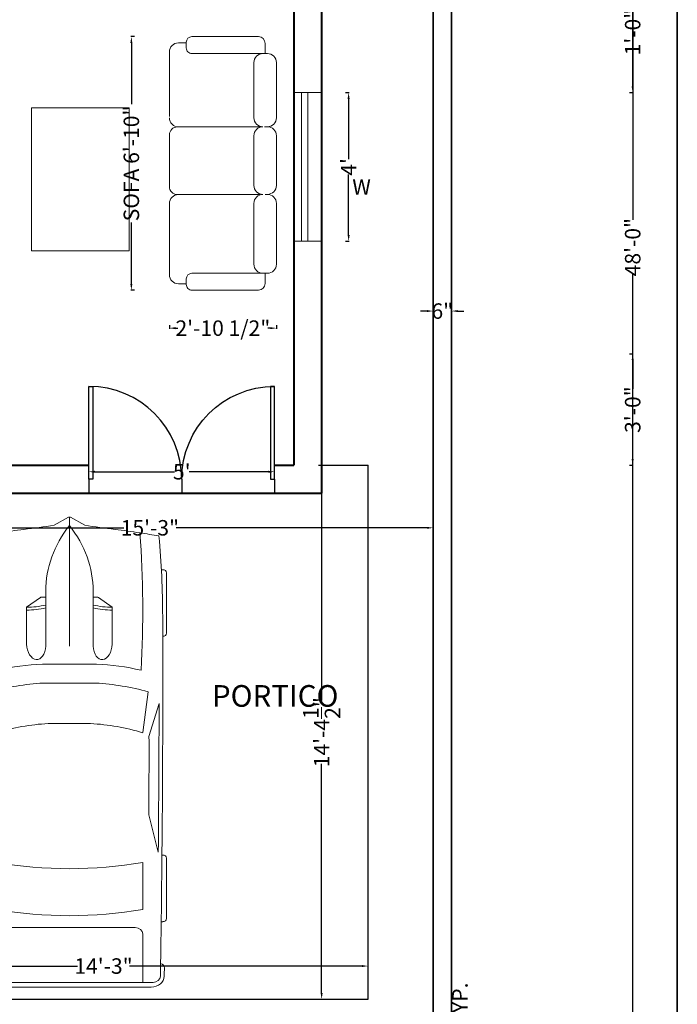
# Model space of a CAD drawing. Units: inches. Extents: x -231 to 349, y -511 to 252.
# Tile 4 of 6: x 136 to 349, y -351 to -33. Entities that reach past the tile are written whole.
import ezdxf

# ---------------------------------------------------------------- set-up
doc = ezdxf.new("R2010")
doc.units = ezdxf.units.IN
doc.header["$MEASUREMENT"] = 0
for name, color, linetype, lineweight in [('A-ANNO-DIMS', 7, 'Continuous', 18), ('A-ANNO-TEXT', 7, 'Continuous', 18), ('A-ANNO-TTLB', 7, 'Continuous', 35), ('A-AREA-IDEN', 7, 'Continuous', 25), ('A-FLOR', 7, 'Continuous', 25), ('A-FURN', 8, 'Continuous', 18), ('A-GLAZ', 177, 'Continuous', 20), ('A-WALL', 7, 'Continuous', 40), ('C-PARK-VEHI', 8, 'Continuous', 13), ('C-PROP', 7, 'Continuous', 35), ('DOOR', 42, 'Continuous', 25)]:
    doc.layers.add(name, color=color, linetype=linetype, lineweight=lineweight)
doc.styles.get("Standard").update_dxf_attribs({"font": 'arial.ttf'})
doc.dimstyles.get("Standard").update_dxf_attribs({"dimtxt": 5, "dimasz": 2, "dimexe": 0.18, "dimexo": 0.0625, "dimgap": 0.09, "dimtad": 0, "dimzin": 0, "dimdsep": 46, "dimlunit": 4, "dimtxsty": 'Standard', "dimcen": 0.09, "dimadec": 0, "dimazin": 0, "dimtfac": 1, "dimtofl": 0, "dimtmove": 0, "dimatfit": 3, "dimfxl": 1, "dimfxlon": 1, "dimtolj": 1, "dimtzin": 0, "dimarcsym": 0})

# ---------------------------------------------------------------- blocks, each defined once
blk = doc.blocks.new('*U2')
for p, q in [((0, 0), (0, -6)), ((40, 0), (40, -6))]:
    blk.add_line(p, q)
blk.add_lwpolyline([(0, 0), (0, 40), (1.75, 40), (1.75, 0)], close=True)
blk.add_arc((0, 0), 40, 0, 90)
blk = doc.blocks.new('*U7')
for p, q in [((21.1, 37.41), (21.1, 36.83)), ((46.55, 38.89), (22.35, 38.89)), ((47.8, 37.39), (47.8, 37.41)), ((87.99, 31.87), (74.76, 35.92)), ((134.31, 35.6), (119.29, 31.78)), ((135.45, 37.07), (135.45, 37.41)), ((136.7, 38.89), (160.9, 38.89)), ((162.15, 37.41), (162.15, 36.77)), ((186.47, -33.5), (186.47, 33.5)), ((188.4, -32.76), (188.4, 32.76)), ((70.03, 31.54), (86.41, 29.35)), ((138.42, 29.35), (157.25, 29.35)), ((186.47, 29.35), (167.01, 29.35)), ((164.52, 26.39), (164.52, -26.39)), ((32.27, 11.63), (36.13, 17.17)), ((36.13, 17.17), (50.94, 17.17)), ((29.77, 9.51), (51.68, 9.51)), ((32.12, 9.51), (32.12, 11.15)), ((58.92, -10.77), (58.92, 10.77)), ((66.55, -10.53), (66.55, 10.53)), ((82.74, 8.5), (82.74, -8.5)), ((186.47, -10.53), (186.47, 10.53)), ((3.27, 6.13), (0.1, 0.41)), ((0, 0), (51.68, 0)), ((0.1, -0.41), (3.27, -6.13)), ((29.77, -9.51), (51.68, -9.51)), ((32.12, -9.51), (32.12, -11.15)), ((32.27, -11.63), (36.13, -17.17)), ((36.13, -17.17), (50.94, -17.17)), ((86.41, -29.35), (70.03, -31.54)), ((157.25, -29.35), (138.42, -29.35)), ((167.01, -29.35), (186.47, -29.35)), ((87.99, -31.87), (74.76, -35.92)), ((134.31, -35.6), (119.29, -31.78)), ((21.1, -37.41), (21.1, -36.83)), ((46.55, -38.89), (22.35, -38.89)), ((47.8, -37.39), (47.8, -37.41)), ((135.45, -37.07), (135.45, -37.41)), ((136.7, -38.89), (160.9, -38.89)), ((162.15, -37.41), (162.15, -36.77))]:
    blk.add_line(p, q)
for centre, major_axis, ratio, start_param, end_param in [((266.03, -27.52), (0, 313.31), 0.842304, 1.367076, 1.39176), ((41.19, -490.86), (0, 528.23), 0.842304, 0.00281, 0.075598), ((22.35, 37.41), (0, -1.48), 0.842304, 3.141593, 4.712389), ((64.48, -10555.62), (0, 10593.03), 0.842304, -0.013397, 0.002797), ((46.55, 37.41), (0, 1.48), 0.842304, -1.570796, 0), ((64.48, -10555.62), (0, -10591.55), 0.842304, 3.133765, 3.140441), ((136.7, 37.41), (0, -1.48), 0.842304, 3.141593, 4.712389), ((160.9, 37.41), (0, 1.48), 0.842304, -1.570796, 0), ((180.63, 35.84), (0, 2.22), 0.842304, -0.013017, 1.249894), ((64.48, -10556.36), (0, 10595.31), 0.842304, -0.013397, -0.013017), ((183.98, 33.5), (0, -2.96), 0.842304, 1.570796, 3.128196), ((183.98, 32.76), (0, -5.25), 0.842304, 1.570796, 3.128196), ((95.79, -3666.35), (0, -3698.24), 0.842304, 3.134049, 3.144098), ((259.18, -27.52), (0, -305.3), 0.842304, 4.528606, 4.561838), ((37.47, -593.96), (0, -623.33), 0.842304, 3.096046, 3.200911), ((134.4, 5.39), (0, -89.78), 0.842304, 4.449482, 4.652344), ((135.29, 5.39), (0, 81.77), 0.842304, 1.245306, 1.50788), ((149.6, 2.8), (0, -79.58), 0.842304, 4.372215, 4.640744), ((17.08, 0), (0, 147.02), 0.842304, 4.511394, 4.913384), ((35.91, 0), (0, 147.02), 0.842304, 4.511394, 4.913384), ((167.01, 26.39), (0, 2.96), 0.842304, 0, 1.570796), ((-204.49, 52.4), (0, -250.96), 0.842304, 1.385369, 1.434372), ((13.04, 17.01), (0, 27.42), 0.842304, 4.435146, 4.718221), ((14.2, 17.01), (0, 27.42), 0.842304, 4.435146, 4.718221), ((50.79, 13.34), (6.34, -0.36), 0.603834, -1.395552, 1.581315), ((29.77, -46.66), (0, 56.17), 0.842304, 0, 0.590319), ((32.75, 11.15), (0, 0.74), 0.842304, 0.879714, 1.570796), ((0.62, 0), (0, -0.74), 0.842304, 4.131459, 5.293319), ((29.77, 46.66), (0, 56.17), 0.842304, 2.551274, 3.141593), ((-204.49, -52.4), (0, 250.96), 0.842304, -1.434372, -1.385369), ((32.75, -11.15), (0, -0.74), 0.842304, 4.712389, 5.403472), ((13.04, -17.01), (0, -27.42), 0.842304, 1.564964, 1.848039), ((14.2, -17.01), (0, -27.42), 0.842304, 1.564964, 1.848039), ((134.4, -5.39), (0, -89.78), 0.842304, -1.510751, -1.307889), ((135.29, -5.39), (0, -81.77), 0.842304, -1.50788, -1.245306), ((149.6, -2.8), (0, -79.58), 0.842304, -1.499151, -1.230623), ((259.18, 27.52), (0, 305.3), 0.842304, 1.721348, 1.754579), ((167.01, -26.39), (0, -2.96), 0.842304, 4.712389, 6.283185), ((266.03, 27.52), (0, 313.31), 0.842304, 1.749832, 1.774517), ((37.47, 593.96), (0, -623.33), 0.842304, -0.059319, 0.045547), ((95.79, 3666.35), (0, -3698.24), 0.842304, -0.002505, 0.007544), ((183.98, -33.5), (0, 2.96), 0.842304, 3.15499, 4.712389), ((183.98, -32.76), (0, -5.25), 0.842304, 0.013397, 1.570796), ((41.19, 490.86), (0, -528.23), 0.842304, -0.075598, -0.00281), ((22.35, -37.41), (0, 1.48), 0.842304, 1.570796, 3.141593), ((64.48, 10555.62), (0, 10593.03), 0.842304, 3.138796, 3.15499), ((46.55, -37.41), (0, -1.48), 0.842304, 0, 1.570796), ((64.48, 10555.62), (0, -10591.55), 0.842304, 0.001152, 0.007828), ((136.7, -37.41), (0, -1.48), 0.842304, -1.570796, 0), ((160.9, -37.41), (0, 1.48), 0.842304, 3.141593, 4.712389), ((180.63, -35.84), (0, -2.22), 0.842304, -1.249894, 0.013017), ((64.48, 10556.36), (0, 10595.31), 0.842304, 3.15461, 3.15499)]:
    blk.add_ellipse(centre, major_axis=major_axis, ratio=ratio, start_param=start_param, end_param=end_param)
at = {"extrusion": (0, 0, -1)}
blk.add_ellipse((50.79, -13.34), major_axis=(6.34, 0.36), ratio=0.603834, start_param=-1.395552, end_param=1.581315, dxfattribs=at)
blk = doc.blocks.new('*D11')
at = {"layer": 'A-ANNO-DIMS', "color": 0, "lineweight": -2, "transparency": 16777216}
for p, q in [((77.92, -339.94), (77.92, -338.76)), ((79.92, -338.94), (154.98, -338.94)), ((246.92, -338.94), (171.86, -338.94)), ((248.92, -339.94), (248.92, -338.76))]:
    blk.add_line(p, q, dxfattribs=at)
at = {"layer": 'A-ANNO-DIMS', "color": 0, "transparency": 16777216}
for points in [[(79.92, -338.61), (79.92, -339.28), (77.92, -338.94)], [(246.92, -338.61), (246.92, -339.28), (248.92, -338.94)]]:
    blk.add_solid(points, dxfattribs=at)
at = {"layer": 'Defpoints', "color": 0, "transparency": 16777216}
for p in [(248.92, -338.94), (77.92, -342.12), (248.92, -342.12)]:
    blk.add_point(p, dxfattribs=at)
at = {"layer": 'A-ANNO-DIMS', "color": 0, "transparency": 16777216, "insert": (163.42, -338.94), "char_height": 5, "attachment_point": 5}
blk.add_mtext('\\A1;14\'-3"', dxfattribs=at)
blk = doc.blocks.new('*D12')
at = {"layer": 'A-ANNO-DIMS', "color": 0, "lineweight": -2, "transparency": 16777216}
for p, q in [((232.92, -177.12), (234.1, -177.12)), ((233.92, -179.12), (233.92, -253.1)), ((233.92, -347.62), (233.92, -273.64)), ((232.92, -349.62), (234.1, -349.62))]:
    blk.add_line(p, q, dxfattribs=at)
at = {"layer": 'A-ANNO-DIMS', "color": 0, "transparency": 16777216}
for points in [[(233.59, -179.12), (234.25, -179.12), (233.92, -177.12)], [(233.59, -347.62), (234.25, -347.62), (233.92, -349.62)]]:
    blk.add_solid(points, dxfattribs=at)
at = {"layer": 'Defpoints', "color": 0, "transparency": 16777216}
for p in [(224.92, -177.12), (233.92, -177.12), (226.59, -349.62)]:
    blk.add_point(p, dxfattribs=at)
at = {"layer": 'A-ANNO-DIMS', "color": 0, "transparency": 16777216, "insert": (233.92, -263.37), "char_height": 5, "attachment_point": 5, "rotation": 90}
blk.add_mtext('\\A1;14\'-4{\\H1x;\\S1/2;}"', dxfattribs=at)
blk = doc.blocks.new('*D13')
at = {"layer": 'A-ANNO-DIMS', "color": 0, "lineweight": -2, "transparency": 16777216}
for p, q in [((269.92, -128.28), (269.92, -127.1)), ((275.92, -128.28), (275.92, -127.1)), ((267.92, -127.28), (265.92, -127.28)), ((277.92, -127.28), (279.92, -127.28))]:
    blk.add_line(p, q, dxfattribs=at)
at = {"layer": 'A-ANNO-DIMS', "color": 0, "transparency": 16777216}
for points in [[(267.92, -126.94), (267.92, -127.61), (269.92, -127.28)], [(277.92, -126.94), (277.92, -127.61), (275.92, -127.28)]]:
    blk.add_solid(points, dxfattribs=at)
at = {"layer": 'Defpoints', "color": 0, "transparency": 16777216}
for p in [(269.92, -128.93), (275.92, -127.28), (275.92, -128.93)]:
    blk.add_point(p, dxfattribs=at)
at = {"layer": 'A-ANNO-DIMS', "color": 0, "transparency": 16777216, "insert": (272.92, -127.28), "char_height": 5, "attachment_point": 5}
blk.add_mtext('\\A1;6"', dxfattribs=at)
blk = doc.blocks.new('*D14')
at = {"layer": 'A-ANNO-DIMS', "color": 0, "lineweight": -2, "transparency": 16777216}
for p, q in [((158.71, -180.21), (158.71, -179.03)), ((160.71, -179.21), (186.32, -179.21)), ((216.71, -179.21), (191.1, -179.21)), ((218.71, -180.21), (218.71, -179.03))]:
    blk.add_line(p, q, dxfattribs=at)
at = {"layer": 'A-ANNO-DIMS', "color": 0, "transparency": 16777216}
for points in [[(160.71, -178.87), (160.71, -179.54), (158.71, -179.21)], [(216.71, -178.87), (216.71, -179.54), (218.71, -179.21)]]:
    blk.add_solid(points, dxfattribs=at)
at = {"layer": 'Defpoints', "color": 0, "transparency": 16777216}
for p in [(218.71, -179.21), (158.71, -183.87), (218.71, -183.87)]:
    blk.add_point(p, dxfattribs=at)
at = {"layer": 'A-ANNO-DIMS', "color": 0, "transparency": 16777216, "insert": (188.71, -179.21), "char_height": 5, "attachment_point": 5}
blk.add_mtext("\\A1;5'", dxfattribs=at)
blk = doc.blocks.new('*D22')
at = {"layer": 'A-ANNO-DIMS', "color": 0, "lineweight": -2, "transparency": 16777216}
for p, q in [((241.64, -56.7), (242.82, -56.7)), ((242.64, -58.7), (242.64, -78.21)), ((242.64, -102.7), (242.64, -83.19)), ((241.64, -104.7), (242.82, -104.7))]:
    blk.add_line(p, q, dxfattribs=at)
at = {"layer": 'A-ANNO-DIMS', "color": 0, "transparency": 16777216}
for points in [[(242.31, -58.7), (242.97, -58.7), (242.64, -56.7)], [(242.31, -102.7), (242.97, -102.7), (242.64, -104.7)]]:
    blk.add_solid(points, dxfattribs=at)
at = {"layer": 'Defpoints', "color": 0, "transparency": 16777216}
for p in [(233.92, -56.7), (242.64, -56.7), (233.92, -104.7)]:
    blk.add_point(p, dxfattribs=at)
at = {"layer": 'A-ANNO-DIMS', "color": 0, "transparency": 16777216, "insert": (242.64, -80.7), "char_height": 5, "attachment_point": 5, "rotation": 90}
blk.add_mtext("\\A1;4'", dxfattribs=at)
blk = doc.blocks.new('A$C0876780F')
for p, q in [((0.72, 0.95), (0.23, 0.95)), ((1.32, 0.95), (0.88, 0.95)), ((1.48, 0.95), (2.02, 0.95)), ((0, 0.79), (0, 0.21)), ((0.15, 0.85), (0.06, 0.85)), ((0.15, 0.87), (0.15, 0.8444)), ((0.15, 0.87), (0.15, 0.85)), ((0.15, 0.21), (0.15, 0.85)), ((0.8, 0.85), (0.8, 0.87)), ((0.8, 0.87), (0.8, 0.85)), ((0.8, 0.87), (0.8, 0.8444)), ((0.8011, 0.8204), (0.8011, 0.08)), ((1.4, 0.85), (1.4, 0.87)), ((1.4, 0.85), (1.4, 0.87)), ((1.4014, 0.08), (1.4014, 0.803)), ((2.1, 0.87), (2.1, 0.85)), ((2.1, 0.87), (2.1, 0.8444)), ((2.1, 0.21), (2.1, 0.85)), ((2.1, 0.85), (2.19, 0.85)), ((2.25, 0.79), (2.25, 0.21)), ((0.72, 0.75), (0.23, 0.75)), ((1.32, 0.75), (0.88, 0.75)), ((1.48, 0.75), (2.02, 0.75)), ((0, 0.21), (0, 0.2)), ((0.15, 0.2), (0.15, 0.25)), ((2.1, 0.2), (2.1, 0.25)), ((2.25, 0.21), (2.25, 0.2)), ((0.05, 0.15), (0.1, 0.15)), ((0.056, 0.15), (0.056, 0.08)), ((2.2, 0.15), (2.15, 0.15)), ((2.194, 0.15), (2.194, 0.08)), ((0.136, 0), (0.7093, 0)), ((0.8011, 0.07), (0.8011, 0.08)), ((0.8711, 0), (1.3314, 0)), ((1.4014, 0.07), (1.4014, 0.08)), ((2.114, 0), (1.48, 0))]:
    blk.add_line(p, q)
for centre, radius, start, end in [((0.23, 0.87), 0.08, 90, 180), ((0.72, 0.87), 0.08, 0, 90), ((0.88, 0.87), 0.08, 90, 180), ((1.32, 0.87), 0.08, 0, 90), ((1.48, 0.87), 0.08, 90, 180), ((2.02, 0.87), 0.08, 0, 90), ((0.06, 0.79), 0.06, 90, 180), ((0.23, 0.83), 0.08, 180, 270), ((0.23, 0.83), 0.08, 180, 270), ((0.72, 0.83), 0.08, 270, 0), ((0.88, 0.83), 0.08, 180, 270), ((0.88, 0.83), 0.08, 180, 270), ((1.32, 0.83), 0.08, 270, 0), ((1.48, 0.83), 0.08, 180, 270), ((2.02, 0.83), 0.08, 270, 0), ((2.02, 0.83), 0.08, 270, 0), ((2.19, 0.79), 0.06, 0, 90), ((0.05, 0.2), 0.05, 180, 270), ((0.1, 0.2), 0.05, 270, 0), ((0.09, 0.21), 0.06, 350.53768, 0), ((2.16, 0.21), 0.06, 180, 189.46232), ((2.15, 0.2), 0.05, 180, 270), ((2.2, 0.2), 0.05, 270, 0), ((0.136, 0.08), 0.08, 180, 270), ((0.7211, 0.08), 0.08, 270, 0), ((0.8711, 0.07), 0.07, 180, 270), ((1.3314, 0.07), 0.07, 270, 0), ((1.4814, 0.08), 0.08, 180, 270), ((2.114, 0.08), 0.08, 270, 0)]:
    blk.add_arc(centre, radius, start, end)
blk = doc.blocks.new('*D27')
at = {"layer": 'A-ANNO-DIMS', "color": 0, "lineweight": -2, "transparency": 16777216}
for p, q in [((86.92, -198.32), (86.92, -197.14)), ((269.92, -198.32), (269.92, -197.14)), ((88.92, -197.32), (169.98, -197.32)), ((267.92, -197.32), (186.86, -197.32))]:
    blk.add_line(p, q, dxfattribs=at)
at = {"layer": 'A-ANNO-DIMS', "color": 0, "transparency": 16777216}
for points in [[(88.92, -196.99), (88.92, -197.66), (86.92, -197.32)], [(267.92, -196.99), (267.92, -197.66), (269.92, -197.32)]]:
    blk.add_solid(points, dxfattribs=at)
at = {"layer": 'Defpoints', "color": 0, "transparency": 16777216}
for p in [(269.92, -197.32), (86.92, -211.86), (269.92, -211.86)]:
    blk.add_point(p, dxfattribs=at)
at = {"layer": 'A-ANNO-DIMS', "color": 0, "transparency": 16777216, "insert": (178.42, -197.32), "char_height": 5, "attachment_point": 5}
blk.add_mtext('\\A1;15\'-3"', dxfattribs=at)
blk = doc.blocks.new('WIN-48IN')
for p, q in [((224.92, -56.7), (233.92, -56.7)), ((227.42, -56.7), (227.42, -104.7)), ((229.42, -56.7), (229.42, -104.7)), ((224.92, -104.7), (233.92, -104.7))]:
    blk.add_line(p, q)
blk = doc.blocks.new('*D33')
at = {"layer": 'A-ANNO-DIMS', "color": 0, "lineweight": -2, "transparency": 16777216}
for p, q in [((278.62, -376.62), (278.62, -374.62)), ((277.62, -376.62), (278.8, -376.62)), ((278.62, -392.62), (278.62, -378.62)), ((277.62, -394.62), (278.8, -394.62))]:
    blk.add_line(p, q, dxfattribs=at)
at = {"layer": 'A-ANNO-DIMS', "color": 0, "transparency": 16777216}
for points in [[(278.29, -378.62), (278.95, -378.62), (278.62, -376.62)], [(278.29, -392.62), (278.95, -392.62), (278.62, -394.62)]]:
    blk.add_solid(points, dxfattribs=at)
at = {"layer": 'Defpoints', "color": 0, "transparency": 16777216}
for p in [(275.92, -376.62), (278.62, -376.62), (275.92, -394.62)]:
    blk.add_point(p, dxfattribs=at)
at = {"layer": 'A-ANNO-DIMS', "color": 0, "transparency": 16777216, "insert": (278.62, -359.53), "char_height": 5, "attachment_point": 5, "rotation": 90}
blk.add_mtext('\\A1;1\'-6" TYP.', dxfattribs=at)
blk = doc.blocks.new('*D42')
at = {"layer": 'A-ANNO-DIMS', "color": 0, "lineweight": -2, "transparency": 16777216}
for p, q in [((173.43, -38.6), (172.25, -38.6)), ((172.43, -40.6), (172.43, -60.41)), ((172.43, -118.52), (172.43, -98.7)), ((173.43, -120.52), (172.25, -120.52))]:
    blk.add_line(p, q, dxfattribs=at)
at = {"layer": 'A-ANNO-DIMS', "color": 0, "transparency": 16777216}
for points in [[(172.1, -40.6), (172.76, -40.6), (172.43, -38.6)], [(172.1, -118.52), (172.76, -118.52), (172.43, -120.52)]]:
    blk.add_solid(points, dxfattribs=at)
at = {"layer": 'Defpoints', "color": 0, "transparency": 16777216}
for p in [(184.72, -38.6), (172.43, -120.52), (184.72, -120.52)]:
    blk.add_point(p, dxfattribs=at)
at = {"layer": 'A-ANNO-DIMS', "color": 0, "transparency": 16777216, "insert": (172.43, -79.56), "char_height": 5, "attachment_point": 5, "rotation": 90}
blk.add_mtext('\\A1;SOFA 6\'-10"', dxfattribs=at)
blk = doc.blocks.new('*D43')
at = {"layer": 'A-ANNO-DIMS', "color": 0, "lineweight": -2, "transparency": 16777216}
for p, q in [((184.72, -131.8), (184.72, -132.98)), ((186.72, -132.8), (187.47, -132.8)), ((217.31, -132.8), (216.56, -132.8)), ((219.31, -131.8), (219.31, -132.98))]:
    blk.add_line(p, q, dxfattribs=at)
at = {"layer": 'A-ANNO-DIMS', "color": 0, "transparency": 16777216}
for points in [[(186.72, -132.47), (186.72, -133.14), (184.72, -132.8)], [(217.31, -132.47), (217.31, -133.14), (219.31, -132.8)]]:
    blk.add_solid(points, dxfattribs=at)
at = {"layer": 'Defpoints', "color": 0, "transparency": 16777216}
for p in [(184.72, -120.52), (219.31, -120.52), (219.31, -132.8)]:
    blk.add_point(p, dxfattribs=at)
at = {"layer": 'A-ANNO-DIMS', "color": 0, "transparency": 16777216, "insert": (202.01, -132.8), "char_height": 5, "attachment_point": 5}
blk.add_mtext('\\A1;2\'-10 1/2"', dxfattribs=at)
blk = doc.blocks.new('*D45')
at = {"layer": 'A-ANNO-DIMS', "color": 0, "lineweight": -2, "transparency": 16777216}
for p, q in [((333.44, 181.38), (334.62, 181.38)), ((334.44, 179.38), (334.44, -97.84)), ((334.44, -392.62), (334.44, -115.4)), ((333.44, -394.62), (334.62, -394.62))]:
    blk.add_line(p, q, dxfattribs=at)
at = {"layer": 'A-ANNO-DIMS', "color": 0, "transparency": 16777216}
for points in [[(334.11, 179.38), (334.78, 179.38), (334.44, 181.38)], [(334.11, -392.62), (334.78, -392.62), (334.44, -394.62)]]:
    blk.add_solid(points, dxfattribs=at)
at = {"layer": 'Defpoints', "color": 0, "transparency": 16777216}
for p in [(275.92, 181.38), (275.92, -394.62), (334.44, -394.62)]:
    blk.add_point(p, dxfattribs=at)
at = {"layer": 'A-ANNO-DIMS', "color": 0, "transparency": 16777216, "insert": (334.44, -106.62), "char_height": 5, "attachment_point": 5, "rotation": 90}
blk.add_mtext('\\A1;48\'-0"', dxfattribs=at)
blk = doc.blocks.new('*D55')
at = {"layer": 'A-ANNO-DIMS', "color": 0, "lineweight": -2, "transparency": 16777216}
for p, q in [((333.44, 64.12), (334.62, 64.12)), ((334.44, 62.12), (334.44, 12.15)), ((334.44, -54.7), (334.44, -4.73)), ((333.44, -56.7), (334.62, -56.7))]:
    blk.add_line(p, q, dxfattribs=at)
at = {"layer": 'A-ANNO-DIMS', "color": 0, "transparency": 16777216}
for points in [[(334.11, 62.12), (334.78, 62.12), (334.44, 64.12)], [(334.11, -54.7), (334.78, -54.7), (334.44, -56.7)]]:
    blk.add_solid(points, dxfattribs=at)
at = {"layer": 'Defpoints', "color": 0, "transparency": 16777216}
for p in [(233.92, 64.12), (233.92, -56.7), (334.44, -56.7)]:
    blk.add_point(p, dxfattribs=at)
at = {"layer": 'A-ANNO-DIMS', "color": 0, "transparency": 16777216, "insert": (334.44, 3.71), "char_height": 5, "attachment_point": 5, "rotation": 90}
blk.add_mtext('\\A1;10\'-1"', dxfattribs=at)
blk = doc.blocks.new('*D57')
at = {"layer": 'A-ANNO-DIMS', "color": 0, "lineweight": -2, "transparency": 16777216}
for p, q in [((216.71, -489.55), (214.71, -489.55)), ((218.71, -488.55), (218.71, -489.73)), ((233.92, -488.55), (233.92, -489.73)), ((235.92, -489.55), (237.92, -489.55))]:
    blk.add_line(p, q, dxfattribs=at)
at = {"layer": 'A-ANNO-DIMS', "color": 0, "transparency": 16777216}
for points in [[(216.71, -489.21), (216.71, -489.88), (218.71, -489.55)], [(235.92, -489.21), (235.92, -489.88), (233.92, -489.55)]]:
    blk.add_solid(points, dxfattribs=at)
at = {"layer": 'Defpoints', "color": 0, "transparency": 16777216}
for p in [(218.71, -186.12), (233.92, -186.12), (233.92, -489.55)]:
    blk.add_point(p, dxfattribs=at)
at = {"layer": 'A-ANNO-DIMS', "color": 0, "transparency": 16777216, "insert": (226.31, -489.55), "char_height": 5, "attachment_point": 5}
blk.add_mtext('\\A1;1\'-3"', dxfattribs=at)
blk = doc.blocks.new('*D64')
at = {"layer": 'A-ANNO-DIMS', "color": 0, "lineweight": -2, "transparency": 16777216}
for p, q in [((333.44, -16.46), (334.62, -16.46)), ((334.44, -18.46), (334.44, -26.62)), ((333.44, -28.62), (334.62, -28.62)), ((334.44, -28.62), (334.44, -30.62))]:
    blk.add_line(p, q, dxfattribs=at)
at = {"layer": 'A-ANNO-DIMS', "color": 0, "transparency": 16777216}
for points in [[(334.11, -18.46), (334.78, -18.46), (334.44, -16.46)], [(334.11, -26.62), (334.78, -26.62), (334.44, -28.62)]]:
    blk.add_solid(points, dxfattribs=at)
at = {"layer": 'Defpoints', "color": 0, "transparency": 16777216}
for p in [(82.42, -16.46), (82.42, -28.62), (334.44, -28.62)]:
    blk.add_point(p, dxfattribs=at)
at = {"layer": 'A-ANNO-DIMS', "color": 0, "transparency": 16777216, "insert": (334.44, -37.12), "char_height": 5, "attachment_point": 5, "rotation": 90}
blk.add_mtext('\\A1;1\'-0"', dxfattribs=at)
blk = doc.blocks.new('*D67')
at = {"layer": 'A-ANNO-DIMS', "color": 0, "lineweight": -2, "transparency": 16777216}
for p, q in [((333.44, -141.12), (334.62, -141.12)), ((334.44, -143.12), (334.44, -152.39)), ((334.44, -175.12), (334.44, -165.85)), ((333.44, -177.12), (334.62, -177.12))]:
    blk.add_line(p, q, dxfattribs=at)
at = {"layer": 'A-ANNO-DIMS', "color": 0, "transparency": 16777216}
for points in [[(334.11, -143.12), (334.78, -143.12), (334.44, -141.12)], [(334.11, -175.12), (334.78, -175.12), (334.44, -177.12)]]:
    blk.add_solid(points, dxfattribs=at)
at = {"layer": 'Defpoints', "color": 0, "transparency": 16777216}
for p in [(-36.08, -141.12), (334.44, -141.12), (-36.08, -177.12)]:
    blk.add_point(p, dxfattribs=at)
at = {"layer": 'A-ANNO-DIMS', "color": 0, "transparency": 16777216, "insert": (334.44, -159.12), "char_height": 5, "attachment_point": 5, "rotation": 90}
blk.add_mtext('\\A1;3\'-0"', dxfattribs=at)

msp = doc.modelspace()

# ---------------------------------------------------------------- linework, layer by layer
at = {"layer": 'A-ANNO-TTLB'}
msp.add_lwpolyline([(-231.158, 252.428), (348.864, 252.428), (348.864, -511.312), (-231.158, -511.312)], close=True, dxfattribs=at)
at = {"layer": 'A-FLOR'}
for p, q in [((233.92, -177.12), (248.92, -177.12)), ((248.92, -349.62), (248.92, -177.12)), ((77.92, -349.62), (248.92, -349.62))]:
    msp.add_line(p, q, dxfattribs=at)
at = {"layer": 'A-FURN'}
msp.add_lwpolyline([(140.189, -61.63), (171.671, -61.63), (171.671, -107.772), (140.189, -107.772)], close=True, dxfattribs=at)
at = {"layer": 'A-WALL'}
for p, q in [((233.92, 142.38), (233.92, -186.12)), ((224.92, 133.38), (224.92, -177.12)), ((77.92, -177.12), (158.708, -177.12)), ((218.708, -177.12), (224.92, -177.12)), ((86.92, -186.12), (233.92, -186.12))]:
    msp.add_line(p, q, dxfattribs=at)
at = {"layer": 'C-PROP'}
for p, q in [((275.92, 181.38), (275.92, -394.62)), ((269.92, 175.38), (269.92, -376.62))]:
    msp.add_line(p, q, dxfattribs=at)

# ---------------------------------------------------------------- block references
at = {"layer": 'A-FURN', "xscale": 36.40817599193578, "yscale": 36.40817599193578, "zscale": 36.40817599193578, "rotation": 270}
msp.add_blockref('A$C0876780F', (184.718, -38.598), dxfattribs=at)
at = {"layer": 'A-GLAZ'}
msp.add_blockref('WIN-48IN', (0, 0), dxfattribs=at)
at = {"layer": 'C-PARK-VEHI', "xscale": 0.806401405747885, "yscale": 0.806401405747885, "zscale": 0.806401405747885, "rotation": 270}
msp.add_blockref('*U7', (152.419, -193.841), dxfattribs=at)
at = {"layer": 'DOOR', "yscale": 0.75, "zscale": 0.75}
for p, xscale in [((158.708, -181.62), 0.75), ((218.708, -181.62), -0.75)]:
    msp.add_blockref('*U2', p, dxfattribs=dict(at, xscale=xscale))

# ---------------------------------------------------------------- texts
at = {"layer": 'A-ANNO-TEXT', "insert": (243.831, -84.673), "char_height": 5, "attachment_point": 1}
msp.add_mtext_dynamic_manual_height_columns('\\A1;W', width=7.82759, gutter_width=1, heights=[0], dxfattribs=at)
at = {"layer": 'A-AREA-IDEN', "insert": (167.584, -248.15), "char_height": 7, "attachment_point": 1}
msp.add_mtext_dynamic_manual_height_columns('\\pxqc;PORTICO', width=102.65834, gutter_width=1, heights=[0], dxfattribs=at)

# ---------------------------------------------------------------- dimensions: what is measured, and where the dimension line sits
at = {"layer": 'A-ANNO-DIMS'}
for base, p1, p2, override, picture, middle in [((334.442, -394.62), (275.92, 181.38), (275.92, -394.62), {"dimdec": 1, "dimlfac": 1, "dimrnd": 0, "dimzin": 1, "dimdsep": 46, "dimlunit": 4, "dimfrac": 2}, '*D45', (334.442, -106.62)), ((334.442, -56.704), (233.92, 64.123), (233.92, -56.704), {"dimdec": 1, "dimlfac": 1, "dimrnd": 0, "dimzin": 1, "dimdsep": 46, "dimlunit": 4, "dimfrac": 2}, '*D55', (334.442, 3.71)), ((334.442, -28.62), (82.42, -16.457), (82.42, -28.62), {"dimdec": 1, "dimlfac": 1, "dimrnd": 0, "dimzin": 1, "dimdsep": 46, "dimlunit": 4, "dimfrac": 2}, '*D64', (334.442, -37.121)), ((242.641, -56.704), (233.92, -104.704), (233.92, -56.704), {"dimclrd": 0, "dimclre": 0, "dimclrt": 0}, '*D22', (242.641, -80.704)), ((334.442, -141.12), (-36.08, -177.12), (-36.08, -141.12), {"dimdec": 1, "dimlfac": 1, "dimrnd": 0, "dimzin": 1, "dimdsep": 46, "dimlunit": 4, "dimfrac": 2}, '*D67', (334.442, -159.12)), ((233.92, -177.12), (226.587, -349.62), (224.92, -177.12), {"dimclrd": 0, "dimclre": 0, "dimclrt": 0}, '*D12', (233.92, -263.37))]:
    dim = msp.add_linear_dim(base=base, p1=p1, p2=p2, angle=90, dimstyle='Standard', override=override, dxfattribs=at)
    dim.commit()
    dim.dimension.update_dxf_attribs({"geometry": picture, "text_midpoint": middle})
for base, p1, p2, angle, text, picture, middle in [((172.43, -120.516), (184.718, -38.598), (184.718, -120.516), 270, 'SOFA <>', '*D42', (172.43, -79.557)), ((278.62, -376.62), (275.92, -394.62), (275.92, -376.62), 90, '<> TYP.', '*D33', (278.62, -359.527))]:
    dim = msp.add_linear_dim(base=base, p1=p1, p2=p2, angle=angle, text=text, dimstyle='Standard', override={"dimdec": 1, "dimlfac": 1, "dimrnd": 0, "dimzin": 1, "dimdsep": 46, "dimlunit": 4, "dimfrac": 2}, dxfattribs=at)
    dim.commit()
    dim.dimension.update_dxf_attribs({"geometry": picture, "text_midpoint": middle})
for base, p1, p2, override, picture, middle in [((219.306, -132.804), (184.718, -120.516), (219.306, -120.516), {"dimdec": 1, "dimlfac": 1, "dimrnd": 0, "dimzin": 1, "dimdsep": 46, "dimlunit": 4, "dimfrac": 2}, '*D43', (202.012, -132.804)), ((275.92, -127.277), (269.92, -128.931), (275.92, -128.931), {"dimclrd": 0, "dimclre": 0, "dimclrt": 0}, '*D13', (272.92, -127.277)), ((218.708, -179.205), (158.708, -183.87), (218.708, -183.87), {"dimclrd": 0, "dimclre": 0, "dimclrt": 0}, '*D14', (188.708, -179.205)), ((233.92, -489.548), (218.708, -186.12), (233.92, -186.12), {"dimdec": 1, "dimlfac": 1, "dimrnd": 0, "dimzin": 1, "dimdsep": 46, "dimlunit": 4, "dimfrac": 2}, '*D57', (226.314, -489.548)), ((269.92, -197.325), (86.92, -211.864), (269.92, -211.864), {"dimclrd": 0, "dimclre": 0, "dimclrt": 0}, '*D27', (178.42, -197.325)), ((248.92, -338.944), (77.92, -342.12), (248.92, -342.12), {"dimclrd": 0, "dimclre": 0, "dimclrt": 0}, '*D11', (163.42, -338.944))]:
    dim = msp.add_linear_dim(base=base, p1=p1, p2=p2, dimstyle='Standard', override=override, dxfattribs=at)
    dim.commit()
    dim.dimension.update_dxf_attribs({"geometry": picture, "text_midpoint": middle})

doc.saveas('drawing.dxf')
